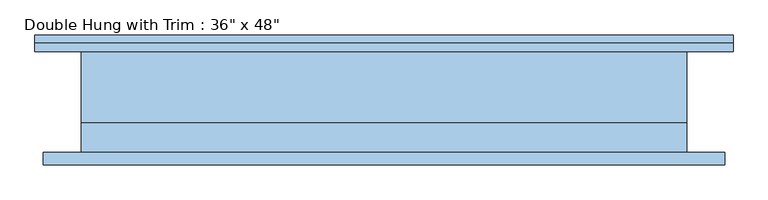
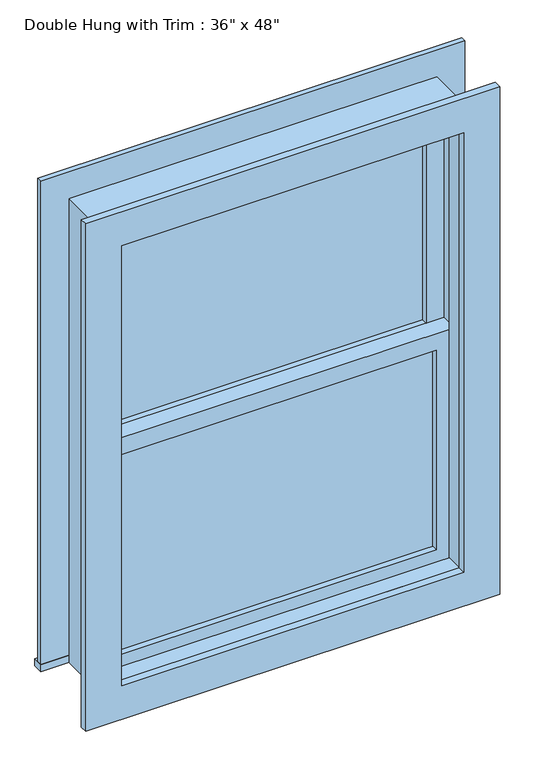
"""IFC4 building model written with IfcOpenShell, lengths in millimetres: window geometry."""

from ifc_helpers import new_model, si_unit, frame, origin, place, context, project, spatial, polyline, outline, extrude, source, transform, mapped, element, save


def window_d24d93a6(model_context):
    return source(origin(), model_context, "Body", "SweptSolid", [
        extrude(outline(polyline([(-393.7, -3.175), (393.7, -3.175), (393.7, -15.875), (-393.7, -15.875), (-393.7, -3.175)])), frame((0.0, 0.0, 977.9), z_axis=(0.0, 0.0, 1.0), x_axis=(1.0, 0.0, 0.0)), (0.0, 0.0, 1.0), 523.875),
        extrude(outline(polyline([(1546.225, -438.15), (933.45, -438.15), (933.45, 438.15), (1546.225, 438.15), (1546.225, -438.15)]), holes=[polyline([(1501.775, -393.7), (1501.775, 393.7), (977.9, 393.7), (977.9, -393.7), (1501.775, -393.7)])]), frame((0.0, -31.75, 0.0), z_axis=(0.0, 1.0, 0.0), x_axis=(0.0, 0.0, 1.0)), (0.0, 0.0, 1.0), 44.45),
        extrude(outline(polyline([(-527.05, 101.6), (527.05, 101.6), (527.05, 76.2), (-527.05, 76.2), (-527.05, 101.6)])), frame((0.0, 0.0, 914.4), z_axis=(0.0, 0.0, 1.0), x_axis=(1.0, 0.0, 0.0)), (0.0, 0.0, 1.0), 19.05),
        extrude(outline(polyline([(2114.55, -438.15), (2114.55, 438.15), (933.45, 438.15), (933.45, 527.05), (2203.45, 527.05), (2203.45, -527.05), (933.45, -527.05), (933.45, -438.15), (2114.55, -438.15)])), frame((0.0, 76.2, 0.0), z_axis=(0.0, 1.0, 0.0), x_axis=(0.0, 0.0, 1.0)), (0.0, 0.0, 1.0), 12.7),
        extrude(outline(polyline([(2190.75, 514.35), (2190.75, -514.35), (857.25, -514.35), (857.25, 514.35), (2190.75, 514.35)]), holes=[polyline([(2101.85, 425.45), (946.15, 425.45), (946.15, -425.45), (2101.85, -425.45), (2101.85, 425.45)])]), frame((0.0, -95.25, 0.0), z_axis=(0.0, 1.0, 0.0), x_axis=(0.0, 0.0, 1.0)), (0.0, 0.0, 1.0), 19.05),
        extrude(outline(polyline([(393.7, 28.575), (-393.7, 28.575), (-393.7, 41.275), (393.7, 41.275), (393.7, 28.575)])), frame((0.0, 0.0, 1546.225), z_axis=(0.0, 0.0, 1.0), x_axis=(1.0, 0.0, 0.0)), (0.0, 0.0, 1.0), 523.875),
        extrude(outline(polyline([(2114.55, -438.15), (1501.775, -438.15), (1501.775, 438.15), (2114.55, 438.15), (2114.55, -438.15)]), holes=[polyline([(2070.1, -393.7), (2070.1, 393.7), (1546.225, 393.7), (1546.225, -393.7), (2070.1, -393.7)])]), frame((0.0, 12.7, 0.0), z_axis=(0.0, 1.0, 0.0), x_axis=(0.0, 0.0, 1.0)), (0.0, 0.0, 1.0), 44.45),
        extrude(outline(polyline([(2133.6, -457.2), (914.4, -457.2), (914.4, 457.2), (2133.6, 457.2), (2133.6, -457.2)]), holes=[polyline([(2101.85, -425.45), (2101.85, 425.45), (946.15, 425.45), (946.15, -425.45), (2101.85, -425.45)])]), frame((0.0, -76.2, 0.0), z_axis=(0.0, 1.0, 0.0), x_axis=(0.0, 0.0, 1.0)), (0.0, 0.0, 1.0), 44.45),
        extrude(outline(polyline([(2133.6, 457.2), (2133.6, -457.2), (914.4, -457.2), (914.4, 457.2), (2133.6, 457.2)]), holes=[polyline([(2114.55, 438.15), (933.45, 438.15), (933.45, -438.15), (2114.55, -438.15), (2114.55, 438.15)])]), frame((0.0, -31.75, 0.0), z_axis=(0.0, 1.0, 0.0), x_axis=(0.0, 0.0, 1.0)), (0.0, 0.0, 1.0), 107.95),
    ])


if __name__ == "__main__":
    model = new_model("IFC4")
    model_context = context("Model", 3, world=origin())
    ifc_project = project(units=[si_unit("LENGTHUNIT", "METRE", prefix="MILLI")], contexts=[model_context])
    site = spatial("IfcSite", under=ifc_project)
    building = spatial("IfcBuilding", under=site)
    placement = place(None, origin())
    window_shape = window_d24d93a6(model_context)
    element("IfcWindow", 1, ObjectType="Double Hung with Trim : 36\" x 48\"", at=placement, inside=building, context=model_context, shape_type="MappedRepresentation", body=[
        mapped(window_shape, transform((0.0, 0.0, 0.0), x_axis=(1.0, 0.0, 0.0), y_axis=(0.0, 1.0, 0.0), z_axis=(0.0, 0.0, 1.0))),
    ])
    save(model, "model.ifc")

# Revit data of these elements
# Type "Double Hung with Trim : 36\" x 48\""
#   Type Mark = "13"
#   Construction Type Id = "GSP4R"
#   Assembly Code = "B2020100"
#   Analytic Construction = "1/8 in Pilkington single glazing"
#   Visual Light Transmittance = 0.9
#   Solar Heat Gain Coefficient = 0.78
#   Heat Transfer Coefficient (U) = 0.6496 BTU/(h·ft²·°F)
#   Height = 4' - 0"
#   Default Sill Height = 3' - 0"
#   Trim Projection - Ext. = 0' - 0 1/2"
#   Trim Projection - Int. = 0' - 0 3/4"
#   Trim Width - Exterior = 0' - 3 1/2"
#   Trim Width - Interior = 0' - 3 1/2"
#   Width = 3' - 0"
#   Window Inset = 0' - 0 3/4"
#   Define Thermal Properties by = 1
#   Glass Pane Material = Glass
#   Sash Material = Sash
#   Trim Exterior Material = Trim
#   Trim Interior Material = Trim
#   Wall Closure = (empty or 0)
# Element 1 (IfcWindow, "Double Hung with Trim : 36\" x 48\"")
#   Materials on its faces: "Sash", "Trim", "Glass"
# Materials
#   "Glass": class "Glass", colour RGB 0 128 192, transparency 0.75, Description = "Soda Lime Glass", Cost = 0
#   "Sash": class "Wood", colour RGB 224 178 126, transparency 0
#   "Trim": class "Wood", colour RGB 224 178 126, transparency 0
